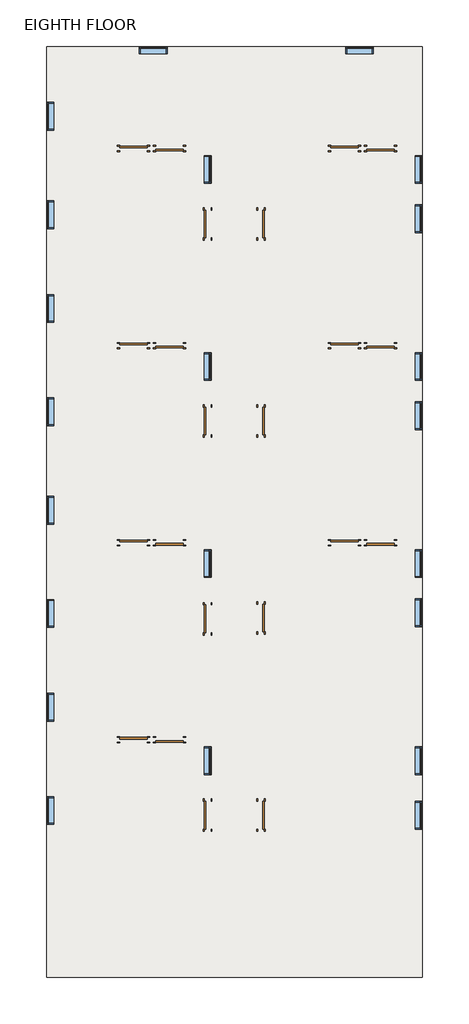
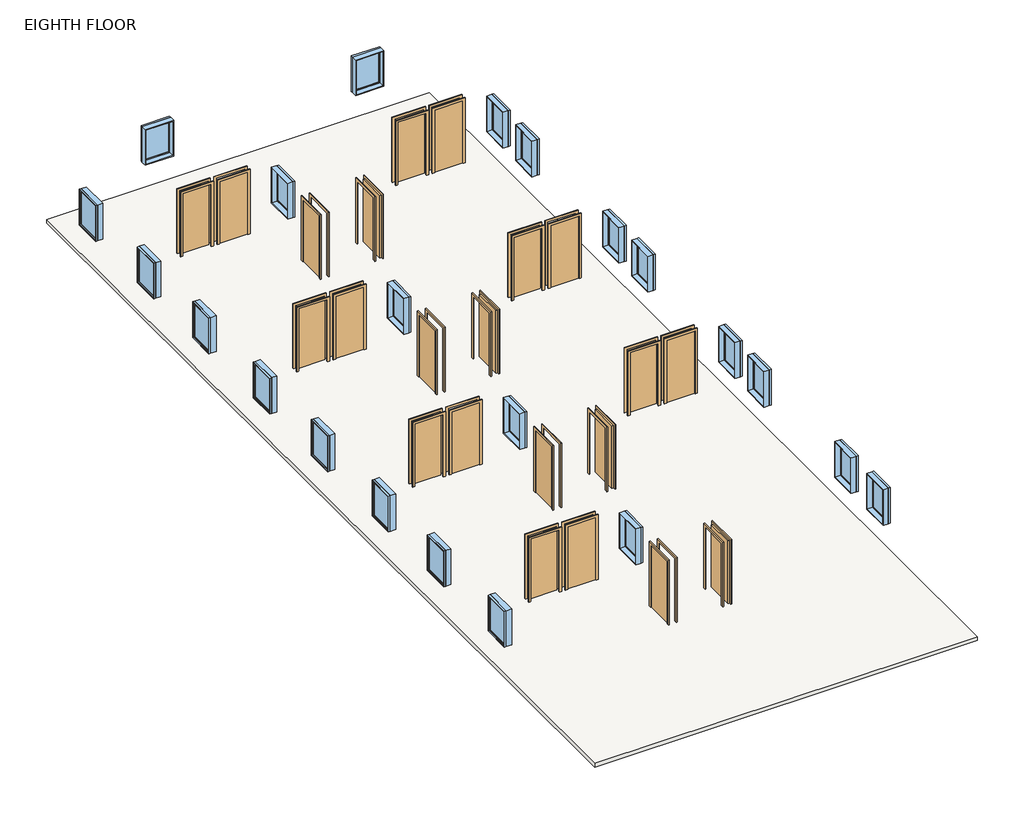
# One storey: 22 doors, 22 windows, 1 slab.
"""IFC4 building model written with IfcOpenShell, lengths in millimetres."""

from ifc_helpers import new_model, si_unit, frame, origin, place, context, project, spatial, polyline, outline, extrude, transform, mapped, element, save
from components import door_686f89d2, door_16372e1c, door_a90ba1ad, door_0ca8825f, window_c1f32544

model = new_model("IFC4")

# Units and contexts
model_context = context("Model", 3, world=origin())
ifc_project = project(units=[si_unit("LENGTHUNIT", "METRE", prefix="MILLI")], contexts=[model_context])

# Site, building, storey
site = spatial("IfcSite", under=ifc_project)
building = spatial("IfcBuilding", under=site)
storey = spatial("IfcBuildingStorey", under=building, Name="EIGHTH FLOOR", Elevation=25603.2)

# Doors
placement = place(None, origin())
door_shape = door_686f89d2(model_context)
element("IfcDoor", 1, ObjectType="Single-Flush : 36\" x 84\"", at=placement, inside=storey, context=model_context, shape_type="MappedRepresentation", body=[
    mapped(door_shape, transform((-9863.5902461, 11952.2710592, 25603.2), x_axis=(-1.0, 0.0, 0.0), y_axis=(0.0, -1.0, 0.0), z_axis=(0.0, 0.0, 1.0))),
])
element("IfcDoor", 2, ObjectType="Single-Flush : 36\" x 84\"", at=placement, inside=storey, context=model_context, shape_type="MappedRepresentation", body=[
    mapped(door_shape, transform((-2929.3902461, 11952.2710592, 25603.2), x_axis=(-1.0, 0.0, 0.0), y_axis=(0.0, -1.0, 0.0), z_axis=(0.0, 0.0, 1.0))),
])
element("IfcDoor", 3, ObjectType="Single-Flush : 36\" x 84\"", at=placement, inside=storey, context=model_context, shape_type="MappedRepresentation", body=[
    mapped(door_shape, transform((-9863.5902461, 5475.2710592, 25603.2), x_axis=(-1.0, 0.0, 0.0), y_axis=(0.0, -1.0, 0.0), z_axis=(0.0, 0.0, 1.0))),
])
element("IfcDoor", 4, ObjectType="Single-Flush : 36\" x 84\"", at=placement, inside=storey, context=model_context, shape_type="MappedRepresentation", body=[
    mapped(door_shape, transform((-2929.3902461, 5475.2710592, 25603.2), x_axis=(-1.0, 0.0, 0.0), y_axis=(0.0, -1.0, 0.0), z_axis=(0.0, 0.0, 1.0))),
])
element("IfcDoor", 5, ObjectType="Single-Flush : 36\" x 84\"", at=placement, inside=storey, context=model_context, shape_type="MappedRepresentation", body=[
    mapped(door_shape, transform((-2929.3902461, -1001.7289408, 25603.2), x_axis=(-1.0, 0.0, 0.0), y_axis=(0.0, -1.0, 0.0), z_axis=(0.0, 0.0, 1.0))),
])
element("IfcDoor", 6, ObjectType="Single-Flush : 36\" x 84\"", at=placement, inside=storey, context=model_context, shape_type="MappedRepresentation", body=[
    mapped(door_shape, transform((-9863.5902461, -1001.7289408, 25603.2), x_axis=(-1.0, 0.0, 0.0), y_axis=(0.0, -1.0, 0.0), z_axis=(0.0, 0.0, 1.0))),
])
element("IfcDoor", 7, ObjectType="Single-Flush : 36\" x 84\"", at=placement, inside=storey, context=model_context, shape_type="MappedRepresentation", body=[
    mapped(door_shape, transform((-9863.5902461, -7478.7289408, 25603.2), x_axis=(-1.0, 0.0, 0.0), y_axis=(0.0, -1.0, 0.0), z_axis=(0.0, 0.0, 1.0))),
])
door_2_shape = door_16372e1c(model_context)
element("IfcDoor", 8, ObjectType="Single-Flush : 36\" x 84\"", at=placement, inside=storey, context=model_context, shape_type="MappedRepresentation", body=[
    mapped(door_2_shape, transform((-8682.4902461, 11952.2710592, 25603.2), x_axis=(-1.0, 0.0, 0.0), y_axis=(0.0, -1.0, 0.0), z_axis=(0.0, 0.0, 1.0))),
])
element("IfcDoor", 9, ObjectType="Single-Flush : 36\" x 84\"", at=placement, inside=storey, context=model_context, shape_type="MappedRepresentation", body=[
    mapped(door_2_shape, transform((-1748.2902461, 11952.2710592, 25603.2), x_axis=(-1.0, 0.0, 0.0), y_axis=(0.0, -1.0, 0.0), z_axis=(0.0, 0.0, 1.0))),
])
element("IfcDoor", 10, ObjectType="Single-Flush : 36\" x 84\"", at=placement, inside=storey, context=model_context, shape_type="MappedRepresentation", body=[
    mapped(door_2_shape, transform((-8682.4902461, 5475.2710592, 25603.2), x_axis=(-1.0, 0.0, 0.0), y_axis=(0.0, -1.0, 0.0), z_axis=(0.0, 0.0, 1.0))),
])
element("IfcDoor", 11, ObjectType="Single-Flush : 36\" x 84\"", at=placement, inside=storey, context=model_context, shape_type="MappedRepresentation", body=[
    mapped(door_2_shape, transform((-1748.2902461, 5475.2710592, 25603.2), x_axis=(-1.0, 0.0, 0.0), y_axis=(0.0, -1.0, 0.0), z_axis=(0.0, 0.0, 1.0))),
])
element("IfcDoor", 12, ObjectType="Single-Flush : 36\" x 84\"", at=placement, inside=storey, context=model_context, shape_type="MappedRepresentation", body=[
    mapped(door_2_shape, transform((-1748.2902461, -1001.7289408, 25603.2), x_axis=(-1.0, 0.0, 0.0), y_axis=(0.0, -1.0, 0.0), z_axis=(0.0, 0.0, 1.0))),
])
element("IfcDoor", 13, ObjectType="Single-Flush : 36\" x 84\"", at=placement, inside=storey, context=model_context, shape_type="MappedRepresentation", body=[
    mapped(door_2_shape, transform((-8682.4902461, -1001.7289408, 25603.2), x_axis=(-1.0, 0.0, 0.0), y_axis=(0.0, -1.0, 0.0), z_axis=(0.0, 0.0, 1.0))),
])
element("IfcDoor", 14, ObjectType="Single-Flush : 36\" x 84\"", at=placement, inside=storey, context=model_context, shape_type="MappedRepresentation", body=[
    mapped(door_2_shape, transform((-8682.4902461, -7478.7289408, 25603.2), x_axis=(-1.0, 0.0, 0.0), y_axis=(0.0, -1.0, 0.0), z_axis=(0.0, 0.0, 1.0))),
])
door_3_shape = door_a90ba1ad(model_context)
element("IfcDoor", 15, ObjectType="Single-Flush : 36\" x 84\"", at=placement, inside=storey, context=model_context, shape_type="MappedRepresentation", body=[
    mapped(door_3_shape, transform((-7425.1902461, 9475.7710592, 25603.2), x_axis=(0.0, -1.0, 0.0), y_axis=(1.0, 0.0, 0.0), z_axis=(0.0, 0.0, 1.0))),
])
element("IfcDoor", 16, ObjectType="Single-Flush : 36\" x 84\"", at=placement, inside=storey, context=model_context, shape_type="MappedRepresentation", body=[
    mapped(door_3_shape, transform((-7425.1902461, -9955.2289408, 25603.2), x_axis=(0.0, -1.0, 0.0), y_axis=(1.0, 0.0, 0.0), z_axis=(0.0, 0.0, 1.0))),
])
element("IfcDoor", 17, ObjectType="Single-Flush : 36\" x 84\"", at=placement, inside=storey, context=model_context, shape_type="MappedRepresentation", body=[
    mapped(door_3_shape, transform((-7425.1902461, -3503.6289408, 25603.2), x_axis=(0.0, -1.0, 0.0), y_axis=(1.0, 0.0, 0.0), z_axis=(0.0, 0.0, 1.0))),
])
element("IfcDoor", 18, ObjectType="Single-Flush : 36\" x 84\"", at=placement, inside=storey, context=model_context, shape_type="MappedRepresentation", body=[
    mapped(door_3_shape, transform((-7425.1902461, 2998.7710592, 25603.2), x_axis=(0.0, -1.0, 0.0), y_axis=(1.0, 0.0, 0.0), z_axis=(0.0, 0.0, 1.0))),
])
door_4_shape = door_0ca8825f(model_context)
element("IfcDoor", 19, ObjectType="Single-Flush : 36\" x 84\"", at=placement, inside=storey, context=model_context, shape_type="MappedRepresentation", body=[
    mapped(door_4_shape, transform((-5672.5902461, 9475.7710592, 25603.2), x_axis=(0.0, -1.0, 0.0), y_axis=(1.0, 0.0, 0.0), z_axis=(0.0, 0.0, 1.0))),
])
element("IfcDoor", 20, ObjectType="Single-Flush : 36\" x 84\"", at=placement, inside=storey, context=model_context, shape_type="MappedRepresentation", body=[
    mapped(door_4_shape, transform((-5672.5902461, -9955.2289408, 25603.2), x_axis=(0.0, -1.0, 0.0), y_axis=(1.0, 0.0, 0.0), z_axis=(0.0, 0.0, 1.0))),
])
element("IfcDoor", 21, ObjectType="Single-Flush : 36\" x 84\"", at=placement, inside=storey, context=model_context, shape_type="MappedRepresentation", body=[
    mapped(door_4_shape, transform((-5672.5902461, -3478.2289408, 25603.2), x_axis=(0.0, -1.0, 0.0), y_axis=(1.0, 0.0, 0.0), z_axis=(0.0, 0.0, 1.0))),
])
element("IfcDoor", 22, ObjectType="Single-Flush : 36\" x 84\"", at=placement, inside=storey, context=model_context, shape_type="MappedRepresentation", body=[
    mapped(door_4_shape, transform((-5672.5902461, 2998.7710592, 25603.2), x_axis=(0.0, -1.0, 0.0), y_axis=(1.0, 0.0, 0.0), z_axis=(0.0, 0.0, 1.0))),
])

# Slab
element("IfcSlab", 23, ObjectType="Generic - 12\"", at=placement, inside=storey, context=model_context, shape_type="SweptSolid", body=[
    extrude(outline(polyline([(-376.6902461, 15305.0710592), (-376.6902461, -15289.2289408), (-12721.0902461, -15289.2289408), (-12721.0902461, 15305.0710592), (-376.6902461, 15305.0710592)])), frame((0.0, 0.0, 25476.2), z_axis=(0.0, 0.0, 1.0), x_axis=(1.0, 0.0, 0.0)), (0.0, 0.0, 1.0), 127.0),
])

# Windows
window_shape = window_c1f32544(model_context)
element("IfcWindow", 24, ObjectType="Fixed : 36\" x 48\"", at=placement, inside=storey, context=model_context, shape_type="MappedRepresentation", body=[
    mapped(window_shape, transform((-9177.7902461, 15190.7710592, 25603.2), x_axis=(1.0, 0.0, 0.0), y_axis=(0.0, 1.0, 0.0), z_axis=(0.0, 0.0, 1.0))),
])
element("IfcWindow", 25, ObjectType="Fixed : 36\" x 48\"", at=placement, inside=storey, context=model_context, shape_type="MappedRepresentation", body=[
    mapped(window_shape, transform((-2395.9902461, 15190.7710592, 25603.2), x_axis=(1.0, 0.0, 0.0), y_axis=(0.0, 1.0, 0.0), z_axis=(0.0, 0.0, 1.0))),
])
element("IfcWindow", 26, ObjectType="Fixed : 36\" x 48\"", at=placement, inside=storey, context=model_context, shape_type="MappedRepresentation", body=[
    mapped(window_shape, transform((-490.9902461, 11228.3710592, 25603.2), x_axis=(0.0, -1.0, 0.0), y_axis=(1.0, 0.0, 0.0), z_axis=(0.0, 0.0, 1.0))),
])
element("IfcWindow", 27, ObjectType="Fixed : 36\" x 48\"", at=placement, inside=storey, context=model_context, shape_type="MappedRepresentation", body=[
    mapped(window_shape, transform((-490.9902461, 4751.3710592, 25603.2), x_axis=(0.0, -1.0, 0.0), y_axis=(1.0, 0.0, 0.0), z_axis=(0.0, 0.0, 1.0))),
])
element("IfcWindow", 28, ObjectType="Fixed : 36\" x 48\"", at=placement, inside=storey, context=model_context, shape_type="MappedRepresentation", body=[
    mapped(window_shape, transform((-490.9902461, -1725.6289408, 25603.2), x_axis=(0.0, -1.0, 0.0), y_axis=(1.0, 0.0, 0.0), z_axis=(0.0, 0.0, 1.0))),
])
element("IfcWindow", 29, ObjectType="Fixed : 36\" x 48\"", at=placement, inside=storey, context=model_context, shape_type="MappedRepresentation", body=[
    mapped(window_shape, transform((-490.9902461, -8202.6289408, 25603.2), x_axis=(0.0, -1.0, 0.0), y_axis=(1.0, 0.0, 0.0), z_axis=(0.0, 0.0, 1.0))),
])
element("IfcWindow", 30, ObjectType="Fixed : 36\" x 48\"", at=placement, inside=storey, context=model_context, shape_type="MappedRepresentation", body=[
    mapped(window_shape, transform((-490.9902461, -9993.3289408, 25603.2), x_axis=(0.0, -1.0, 0.0), y_axis=(1.0, 0.0, 0.0), z_axis=(0.0, 0.0, 1.0))),
])
element("IfcWindow", 31, ObjectType="Fixed : 36\" x 48\"", at=placement, inside=storey, context=model_context, shape_type="MappedRepresentation", body=[
    mapped(window_shape, transform((-490.9902461, -3344.8789408, 25603.2), x_axis=(0.0, -1.0, 0.0), y_axis=(1.0, 0.0, 0.0), z_axis=(0.0, 0.0, 1.0))),
])
element("IfcWindow", 32, ObjectType="Fixed : 36\" x 48\"", at=placement, inside=storey, context=model_context, shape_type="MappedRepresentation", body=[
    mapped(window_shape, transform((-490.9902461, 3132.1210592, 25603.2), x_axis=(0.0, -1.0, 0.0), y_axis=(1.0, 0.0, 0.0), z_axis=(0.0, 0.0, 1.0))),
])
element("IfcWindow", 33, ObjectType="Fixed : 36\" x 48\"", at=placement, inside=storey, context=model_context, shape_type="MappedRepresentation", body=[
    mapped(window_shape, transform((-490.9902461, 9609.1210592, 25603.2), x_axis=(0.0, -1.0, 0.0), y_axis=(1.0, 0.0, 0.0), z_axis=(0.0, 0.0, 1.0))),
])
element("IfcWindow", 34, ObjectType="Fixed : 36\" x 48\"", at=placement, inside=storey, context=model_context, shape_type="MappedRepresentation", body=[
    mapped(window_shape, transform((-12606.7902461, 9818.6710592, 25603.2), x_axis=(0.0, 1.0, 0.0), y_axis=(-1.0, 0.0, 0.0), z_axis=(0.0, 0.0, 1.0))),
])
element("IfcWindow", 35, ObjectType="Fixed : 36\" x 48\"", at=placement, inside=storey, context=model_context, shape_type="MappedRepresentation", body=[
    mapped(window_shape, transform((-12606.7902461, 13057.1710592, 25603.2), x_axis=(0.0, 1.0, 0.0), y_axis=(-1.0, 0.0, 0.0), z_axis=(0.0, 0.0, 1.0))),
])
element("IfcWindow", 36, ObjectType="Fixed : 36\" x 48\"", at=placement, inside=storey, context=model_context, shape_type="MappedRepresentation", body=[
    mapped(window_shape, transform((-12606.7902461, 6732.5710592, 25603.2), x_axis=(0.0, 1.0, 0.0), y_axis=(-1.0, 0.0, 0.0), z_axis=(0.0, 0.0, 1.0))),
])
element("IfcWindow", 37, ObjectType="Fixed : 36\" x 48\"", at=placement, inside=storey, context=model_context, shape_type="MappedRepresentation", body=[
    mapped(window_shape, transform((-12606.7902461, 3341.6710592, 25603.2), x_axis=(0.0, 1.0, 0.0), y_axis=(-1.0, 0.0, 0.0), z_axis=(0.0, 0.0, 1.0))),
])
element("IfcWindow", 38, ObjectType="Fixed : 36\" x 48\"", at=placement, inside=storey, context=model_context, shape_type="MappedRepresentation", body=[
    mapped(window_shape, transform((-12606.7902461, 103.1710592, 25603.2), x_axis=(0.0, 1.0, 0.0), y_axis=(-1.0, 0.0, 0.0), z_axis=(0.0, 0.0, 1.0))),
])
element("IfcWindow", 39, ObjectType="Fixed : 36\" x 48\"", at=placement, inside=storey, context=model_context, shape_type="MappedRepresentation", body=[
    mapped(window_shape, transform((-12606.7902461, -3287.7289408, 25603.2), x_axis=(0.0, 1.0, 0.0), y_axis=(-1.0, 0.0, 0.0), z_axis=(0.0, 0.0, 1.0))),
])
element("IfcWindow", 40, ObjectType="Fixed : 36\" x 48\"", at=placement, inside=storey, context=model_context, shape_type="MappedRepresentation", body=[
    mapped(window_shape, transform((-12606.7902461, -6373.8289408, 25603.2), x_axis=(0.0, 1.0, 0.0), y_axis=(-1.0, 0.0, 0.0), z_axis=(0.0, 0.0, 1.0))),
])
element("IfcWindow", 41, ObjectType="Fixed : 36\" x 48\"", at=placement, inside=storey, context=model_context, shape_type="MappedRepresentation", body=[
    mapped(window_shape, transform((-12606.7902461, -9764.7289408, 25603.2), x_axis=(0.0, 1.0, 0.0), y_axis=(-1.0, 0.0, 0.0), z_axis=(0.0, 0.0, 1.0))),
])
element("IfcWindow", 42, ObjectType="Fixed : 36\" x 48\"", at=placement, inside=storey, context=model_context, shape_type="MappedRepresentation", body=[
    mapped(window_shape, transform((-7425.1902461, -8202.6289408, 25603.2), x_axis=(0.0, -1.0, 0.0), y_axis=(1.0, 0.0, 0.0), z_axis=(0.0, 0.0, 1.0))),
])
element("IfcWindow", 43, ObjectType="Fixed : 36\" x 48\"", at=placement, inside=storey, context=model_context, shape_type="MappedRepresentation", body=[
    mapped(window_shape, transform((-7425.1902461, -1725.6289408, 25603.2), x_axis=(0.0, -1.0, 0.0), y_axis=(1.0, 0.0, 0.0), z_axis=(0.0, 0.0, 1.0))),
])
element("IfcWindow", 44, ObjectType="Fixed : 36\" x 48\"", at=placement, inside=storey, context=model_context, shape_type="MappedRepresentation", body=[
    mapped(window_shape, transform((-7425.1902461, 4751.3710592, 25603.2), x_axis=(0.0, -1.0, 0.0), y_axis=(1.0, 0.0, 0.0), z_axis=(0.0, 0.0, 1.0))),
])
element("IfcWindow", 45, ObjectType="Fixed : 36\" x 48\"", at=placement, inside=storey, context=model_context, shape_type="MappedRepresentation", body=[
    mapped(window_shape, transform((-7425.1902461, 11228.3710592, 25603.2), x_axis=(0.0, -1.0, 0.0), y_axis=(1.0, 0.0, 0.0), z_axis=(0.0, 0.0, 1.0))),
])

save(model, "model.ifc")

# Revit data of these elements
# Type "Single-Flush : 36\" x 84\""
#   Type Mark = "1"
#   Construction Type Id = "MDOOR"
#   Assembly Code = "C1020"
#   Analytic Construction = "Metal"
#   Thickness = 0' - 2"
#   Heat Transfer Coefficient (U) = 0.651978 BTU/(h·ft²·°F)
#   Height = 7' - 0"
#   Trim Projection Ext = 0' - 1"
#   Trim Projection Int = 0' - 1"
#   Trim Width = 0' - 3"
#   Width = 3' - 0"
#   Define Thermal Properties by = 1
#   Door Material = Door - Panel
#   Frame Material = Door - Frame
#   Visual Light Transmittance = 0
#   Solar Heat Gain Coefficient = 0
#   Function = (empty or 0)
#   Wall Closure = (empty or 0)
# Type "Generic - 12\""
#   Assembly Code = "B1010"
#   Function = 0
#   Layers, outside or top first: 0' - 5" no material (function 1)
# Type "Fixed : 36\" x 48\""
#   Type Mark = "1"
#   Construction Type Id = "GSP4R"
#   Assembly Code = "B2020100"
#   Analytic Construction = "1/8 in Pilkington single glazing"
#   Visual Light Transmittance = 0.9
#   Solar Heat Gain Coefficient = 0.78
#   Heat Transfer Coefficient (U) = 0.6496 BTU/(h·ft²·°F)
#   Height = 4' - 0"
#   Default Sill Height = 3' - 0"
#   Width = 3' - 0"
#   Window Inset = 0' - 0 3/4"
#   Define Thermal Properties by = 1
#   Glass Pane Material = Glass
#   Sash Material = Sash
#   Wall Closure = (empty or 0)
# Elements 1, 2, 3, 4, 5, 6, 7, 8, 9, 10, 11, 12, 13, 14, 15, 16, 17, 18, 19, 20, 21, 22 (IfcDoor, "Single-Flush : 36\" x 84\"")
#   Phase Created = New Construction
#   Materials on its faces: "Door - Frame", "Door - Panel"
# Element 23 (IfcSlab, "Generic - 12\"")
#   Height Offset From Level = 0' - 0"
#   Phase Created = New Construction
#   Materials on its faces: "Default Floor"
# Element 24 (IfcWindow, "Fixed : 36\" x 48\"")
#   Mark = "183"
#   Phase Created = New Construction
#   Materials on its faces: "Sash", "Glass"
# Element 25 (IfcWindow, "Fixed : 36\" x 48\"")
#   Mark = "184"
#   Phase Created = New Construction
#   Materials on its faces: "Sash", "Glass"
# Element 26 (IfcWindow, "Fixed : 36\" x 48\"")
#   Mark = "185"
#   Phase Created = New Construction
#   Materials on its faces: "Sash", "Glass"
# Element 27 (IfcWindow, "Fixed : 36\" x 48\"")
#   Mark = "186"
#   Phase Created = New Construction
#   Materials on its faces: "Sash", "Glass"
# Element 28 (IfcWindow, "Fixed : 36\" x 48\"")
#   Mark = "187"
#   Phase Created = New Construction
#   Materials on its faces: "Sash", "Glass"
# Element 29 (IfcWindow, "Fixed : 36\" x 48\"")
#   Mark = "188"
#   Phase Created = New Construction
#   Materials on its faces: "Sash", "Glass"
# Element 30 (IfcWindow, "Fixed : 36\" x 48\"")
#   Mark = "189"
#   Phase Created = New Construction
#   Materials on its faces: "Sash", "Glass"
# Element 31 (IfcWindow, "Fixed : 36\" x 48\"")
#   Mark = "190"
#   Phase Created = New Construction
#   Materials on its faces: "Sash", "Glass"
# Element 32 (IfcWindow, "Fixed : 36\" x 48\"")
#   Mark = "191"
#   Phase Created = New Construction
#   Materials on its faces: "Sash", "Glass"
# Element 33 (IfcWindow, "Fixed : 36\" x 48\"")
#   Mark = "192"
#   Phase Created = New Construction
#   Materials on its faces: "Sash", "Glass"
# Element 34 (IfcWindow, "Fixed : 36\" x 48\"")
#   Mark = "193"
#   Phase Created = New Construction
#   Materials on its faces: "Sash", "Glass"
# Element 35 (IfcWindow, "Fixed : 36\" x 48\"")
#   Mark = "194"
#   Phase Created = New Construction
#   Materials on its faces: "Sash", "Glass"
# Element 36 (IfcWindow, "Fixed : 36\" x 48\"")
#   Mark = "195"
#   Phase Created = New Construction
#   Materials on its faces: "Sash", "Glass"
# Element 37 (IfcWindow, "Fixed : 36\" x 48\"")
#   Mark = "196"
#   Phase Created = New Construction
#   Materials on its faces: "Sash", "Glass"
# Element 38 (IfcWindow, "Fixed : 36\" x 48\"")
#   Mark = "197"
#   Phase Created = New Construction
#   Materials on its faces: "Sash", "Glass"
# Element 39 (IfcWindow, "Fixed : 36\" x 48\"")
#   Mark = "198"
#   Phase Created = New Construction
#   Materials on its faces: "Sash", "Glass"
# Element 40 (IfcWindow, "Fixed : 36\" x 48\"")
#   Mark = "199"
#   Phase Created = New Construction
#   Materials on its faces: "Sash", "Glass"
# Element 41 (IfcWindow, "Fixed : 36\" x 48\"")
#   Mark = "200"
#   Phase Created = New Construction
#   Materials on its faces: "Sash", "Glass"
# Element 42 (IfcWindow, "Fixed : 36\" x 48\"")
#   Mark = "201"
#   Phase Created = New Construction
#   Materials on its faces: "Sash", "Glass"
# Element 43 (IfcWindow, "Fixed : 36\" x 48\"")
#   Mark = "202"
#   Phase Created = New Construction
#   Materials on its faces: "Sash", "Glass"
# Element 44 (IfcWindow, "Fixed : 36\" x 48\"")
#   Mark = "203"
#   Phase Created = New Construction
#   Materials on its faces: "Sash", "Glass"
# Element 45 (IfcWindow, "Fixed : 36\" x 48\"")
#   Mark = "204"
#   Phase Created = New Construction
#   Materials on its faces: "Sash", "Glass"
# Materials
#   "Door - Panel": class "Wood", colour RGB 210 159 95, transparency 0
#   "Door - Frame": colour RGB 118 70 51, transparency 0
#   "Glass": class "Glass", colour RGB 0 128 192, transparency 0.75, Description = "Soda Lime Glass", Cost = 0
#   "Sash": class "Wood", colour RGB 224 178 126, transparency 0
#   "Default Floor": colour RGB 128 128 128, transparency 0
